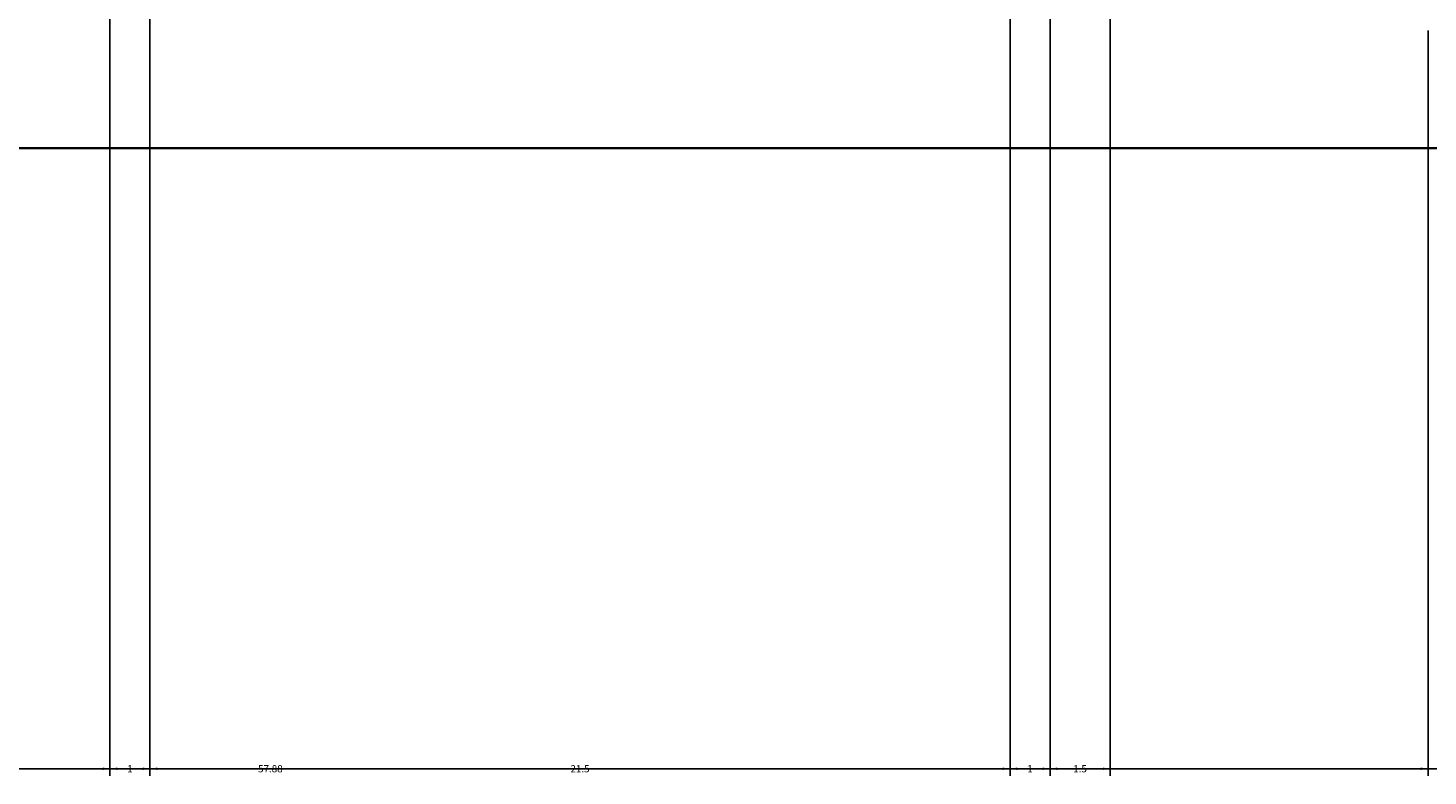
# Model space of a CAD drawing. Units: inches. Extents: x -6 to 289, y -8 to 323.
# Tile 30 of 107: x 209 to 244, y -8 to 10. Entities that reach past the tile are written whole.
import ezdxf

# ---------------------------------------------------------------- set-up
doc = ezdxf.new("R2010")
doc.units = ezdxf.units.IN
doc.header["$MEASUREMENT"] = 0
for name, color, linetype, lineweight in [('A-ANNO-DIMS', 2, 'Continuous', 18), ('A-DOOR', 3, 'Continuous', 25), ('A-ELEV', 7, 'Continuous', 35)]:
    doc.layers.add(name, color=color, linetype=linetype, lineweight=lineweight)
doc.styles.get("Standard").update_dxf_attribs({"font": 'arial.ttf'})
doc.dimstyles.get("Standard").update_dxf_attribs({"dimtxt": 0.18, "dimasz": 0.18, "dimexe": 0.18, "dimexo": 0.0625, "dimgap": 0.09, "dimtad": 0, "dimtih": 1, "dimtoh": 1, "dimdec": 4, "dimzin": 0, "dimdsep": 46, "dimtxsty": 'Standard', "dimcen": 0.09, "dimadec": 0, "dimazin": 0, "dimtfac": 1, "dimtdec": 4, "dimtofl": 0, "dimtmove": 0, "dimatfit": 3, "dimfxl": 1, "dimtolj": 1, "dimtzin": 0, "dimarcsym": 0})

# ---------------------------------------------------------------- blocks, each defined once
blk = doc.blocks.new('*D16')
at = {"layer": 'A-ANNO-DIMS', "color": 0, "lineweight": -2, "transparency": 16777216}
for p, q in [((9.943, 68.37), (9.943, -8.391)), ((272.973, 68.37), (272.973, -8.391)), ((10.123, -8.211), (140.993, -8.211)), ((272.793, -8.211), (141.923, -8.211))]:
    blk.add_line(p, q, dxfattribs=at)
at = {"layer": 'A-ANNO-DIMS', "color": 0, "transparency": 16777216}
for points in [[(10.123, -8.181), (10.123, -8.241), (9.943, -8.211)], [(272.793, -8.181), (272.793, -8.241), (272.973, -8.211)]]:
    blk.add_solid(points, dxfattribs=at)
at = {"layer": 'Defpoints', "color": 0, "transparency": 16777216}
for p in [(9.943, 68.432), (272.973, 68.432), (272.973, -8.211)]:
    blk.add_point(p, dxfattribs=at)
at = {"layer": 'A-ANNO-DIMS', "color": 0, "transparency": 16777216, "insert": (141.458, -8.211), "char_height": 0.18, "attachment_point": 5}
blk.add_mtext('\\A1;263.03', dxfattribs=at)
blk = doc.blocks.new('*D42')
at = {"layer": 'A-ANNO-DIMS', "color": 0, "lineweight": -2, "transparency": 16777216}
for p, q in [((190.792, 224.326), (190.792, -8.391)), ((211.292, 224.326), (211.292, -8.391)), ((190.972, -8.211), (200.716, -8.211)), ((211.112, -8.211), (201.368, -8.211))]:
    blk.add_line(p, q, dxfattribs=at)
at = {"layer": 'A-ANNO-DIMS', "color": 0, "transparency": 16777216}
for points in [[(190.972, -8.181), (190.972, -8.241), (190.792, -8.211)], [(211.112, -8.181), (211.112, -8.241), (211.292, -8.211)]]:
    blk.add_solid(points, dxfattribs=at)
at = {"layer": 'Defpoints', "color": 0, "transparency": 16777216}
for p in [(190.792, 224.389), (211.292, 224.389), (211.292, -8.211)]:
    blk.add_point(p, dxfattribs=at)
at = {"layer": 'A-ANNO-DIMS', "color": 0, "transparency": 16777216, "insert": (201.042, -8.211), "char_height": 0.18, "attachment_point": 5}
blk.add_mtext('\\A1;20.5', dxfattribs=at)
blk = doc.blocks.new('*D43')
at = {"layer": 'A-ANNO-DIMS', "color": 0, "lineweight": -2, "transparency": 16777216}
for p, q in [((211.292, 224.326), (211.292, -8.391)), ((212.292, 224.326), (212.292, -8.391)), ((211.472, -8.211), (211.669, -8.211)), ((212.112, -8.211), (211.915, -8.211))]:
    blk.add_line(p, q, dxfattribs=at)
at = {"layer": 'A-ANNO-DIMS', "color": 0, "transparency": 16777216}
for points in [[(211.472, -8.181), (211.472, -8.241), (211.292, -8.211)], [(212.112, -8.181), (212.112, -8.241), (212.292, -8.211)]]:
    blk.add_solid(points, dxfattribs=at)
at = {"layer": 'Defpoints', "color": 0, "transparency": 16777216}
for p in [(211.292, 224.389), (212.292, 224.389), (212.292, -8.211)]:
    blk.add_point(p, dxfattribs=at)
at = {"layer": 'A-ANNO-DIMS', "color": 0, "transparency": 16777216, "insert": (211.792, -8.211), "char_height": 0.18, "attachment_point": 5}
blk.add_mtext('\\A1;1', dxfattribs=at)
blk = doc.blocks.new('*D44')
at = {"layer": 'A-ANNO-DIMS', "color": 0, "lineweight": -2, "transparency": 16777216}
for p, q in [((212.292, 224.326), (212.292, -8.391)), ((233.792, 224.326), (233.792, -8.391)), ((212.472, -8.211), (222.716, -8.211)), ((233.612, -8.211), (223.368, -8.211))]:
    blk.add_line(p, q, dxfattribs=at)
at = {"layer": 'A-ANNO-DIMS', "color": 0, "transparency": 16777216}
for points in [[(212.472, -8.181), (212.472, -8.241), (212.292, -8.211)], [(233.612, -8.181), (233.612, -8.241), (233.792, -8.211)]]:
    blk.add_solid(points, dxfattribs=at)
at = {"layer": 'Defpoints', "color": 0, "transparency": 16777216}
for p in [(212.292, 224.389), (233.792, 224.389), (233.792, -8.211)]:
    blk.add_point(p, dxfattribs=at)
at = {"layer": 'A-ANNO-DIMS', "color": 0, "transparency": 16777216, "insert": (223.042, -8.211), "char_height": 0.18, "attachment_point": 5}
blk.add_mtext('\\A1;21.5', dxfattribs=at)
blk = doc.blocks.new('*D45')
at = {"layer": 'A-ANNO-DIMS', "color": 0, "lineweight": -2, "transparency": 16777216}
for p, q in [((234.792, 225.326), (234.792, -8.391)), ((233.792, 224.326), (233.792, -8.391)), ((233.972, -8.211), (234.169, -8.211)), ((234.612, -8.211), (234.415, -8.211))]:
    blk.add_line(p, q, dxfattribs=at)
at = {"layer": 'A-ANNO-DIMS', "color": 0, "transparency": 16777216}
for points in [[(233.972, -8.181), (233.972, -8.241), (233.792, -8.211)], [(234.612, -8.181), (234.612, -8.241), (234.792, -8.211)]]:
    blk.add_solid(points, dxfattribs=at)
at = {"layer": 'Defpoints', "color": 0, "transparency": 16777216}
for p in [(234.792, 225.389), (233.792, 224.389), (234.792, -8.211)]:
    blk.add_point(p, dxfattribs=at)
at = {"layer": 'A-ANNO-DIMS', "color": 0, "transparency": 16777216, "insert": (234.292, -8.211), "char_height": 0.18, "attachment_point": 5}
blk.add_mtext('\\A1;1', dxfattribs=at)
blk = doc.blocks.new('*D46')
at = {"layer": 'A-ANNO-DIMS', "color": 0, "lineweight": -2, "transparency": 16777216}
for p, q in [((236.292, 226.826), (236.292, -8.391)), ((234.792, 225.326), (234.792, -8.391)), ((234.972, -8.211), (235.296, -8.211)), ((236.112, -8.211), (235.788, -8.211))]:
    blk.add_line(p, q, dxfattribs=at)
at = {"layer": 'A-ANNO-DIMS', "color": 0, "transparency": 16777216}
for points in [[(234.972, -8.181), (234.972, -8.241), (234.792, -8.211)], [(236.112, -8.181), (236.112, -8.241), (236.292, -8.211)]]:
    blk.add_solid(points, dxfattribs=at)
at = {"layer": 'Defpoints', "color": 0, "transparency": 16777216}
for p in [(236.292, 226.889), (234.792, 225.389), (236.292, -8.211)]:
    blk.add_point(p, dxfattribs=at)
at = {"layer": 'A-ANNO-DIMS', "color": 0, "transparency": 16777216, "insert": (235.542, -8.211), "char_height": 0.18, "attachment_point": 5}
blk.add_mtext('\\A1;1.5', dxfattribs=at)
blk = doc.blocks.new('*D70')
at = {"layer": 'A-ANNO-DIMS', "color": 0, "lineweight": -2, "transparency": 16777216}
for p, q in [((186.36, 10.226), (186.36, -8.391)), ((244.241, 10.226), (244.241, -8.391)), ((186.54, -8.211), (214.907, -8.211)), ((244.061, -8.211), (215.694, -8.211))]:
    blk.add_line(p, q, dxfattribs=at)
at = {"layer": 'A-ANNO-DIMS', "color": 0, "transparency": 16777216}
for points in [[(186.54, -8.181), (186.54, -8.241), (186.36, -8.211)], [(244.061, -8.181), (244.061, -8.241), (244.241, -8.211)]]:
    blk.add_solid(points, dxfattribs=at)
at = {"layer": 'Defpoints', "color": 0, "transparency": 16777216}
for p in [(186.36, 10.289), (244.241, 10.289), (244.241, -8.211)]:
    blk.add_point(p, dxfattribs=at)
at = {"layer": 'A-ANNO-DIMS', "color": 0, "transparency": 16777216, "insert": (215.301, -8.211), "char_height": 0.18, "attachment_point": 5}
blk.add_mtext('\\A1;57.88', dxfattribs=at)

msp = doc.modelspace()

# ---------------------------------------------------------------- linework, layer by layer
at = {"layer": 'A-DOOR'}
msp.add_lwpolyline([(121.008, 51.0851), (247.2408, 51.0851), (247.2408, 7.2888), (121.008, 7.2888)], close=True, dxfattribs=at)
at = {"layer": 'A-ELEV'}
msp.add_line((19.1638, 7.2888), (271.1638, 7.2888), dxfattribs=at)

# ---------------------------------------------------------------- dimensions: what is measured, and where the dimension line sits
at = {"layer": 'A-ANNO-DIMS'}
for base, p1, p2, override, picture, middle in [((236.2918, -8.2112), (234.7918, 225.3887), (236.2918, 226.8887), {"dimdec": 1, "dimlfac": 1, "dimrnd": 0, "dimzin": 0, "dimdsep": 46, "dimlunit": 2}, '*D46', (235.5418, -8.2112)), ((234.7918, -8.2112), (233.7918, 224.3887), (234.7918, 225.3887), {"dimdec": 0, "dimlfac": 1, "dimrnd": 0, "dimzin": 0, "dimdsep": 46, "dimlunit": 2}, '*D45', (234.2918, -8.2112)), ((211.2918, -8.2112), (190.7918, 224.3887), (211.2918, 224.3887), {"dimdec": 1, "dimlfac": 1, "dimrnd": 0, "dimzin": 0, "dimdsep": 46, "dimlunit": 2}, '*D42', (201.0418, -8.2112)), ((212.2918, -8.2112), (211.2918, 224.3887), (212.2918, 224.3887), {"dimdec": 0, "dimlfac": 1, "dimrnd": 0, "dimzin": 0, "dimdsep": 46, "dimlunit": 2}, '*D43', (211.7918, -8.2112)), ((233.7918, -8.2112), (212.2918, 224.3887), (233.7918, 224.3887), {"dimdec": 1, "dimlfac": 1, "dimrnd": 0, "dimzin": 0, "dimdsep": 46, "dimlunit": 2}, '*D44', (223.0418, -8.2112)), ((272.9733, -8.2112), (9.943, 68.4322), (272.9733, 68.4322), {"dimdec": 2, "dimlfac": 1, "dimrnd": 0, "dimzin": 0, "dimdsep": 46, "dimlunit": 2}, '*D16', (141.4581, -8.2112)), ((244.2408, -8.2112), (186.3604, 10.2888), (244.2408, 10.2888), {"dimdec": 2, "dimlfac": 1, "dimrnd": 0, "dimzin": 0, "dimdsep": 46, "dimlunit": 2}, '*D70', (215.3006, -8.2112))]:
    dim = msp.add_linear_dim(base=base, p1=p1, p2=p2, dimstyle='Standard', override=override, dxfattribs=at)
    dim.commit()
    dim.dimension.update_dxf_attribs({"geometry": picture, "text_midpoint": middle})

doc.saveas('drawing.dxf')
